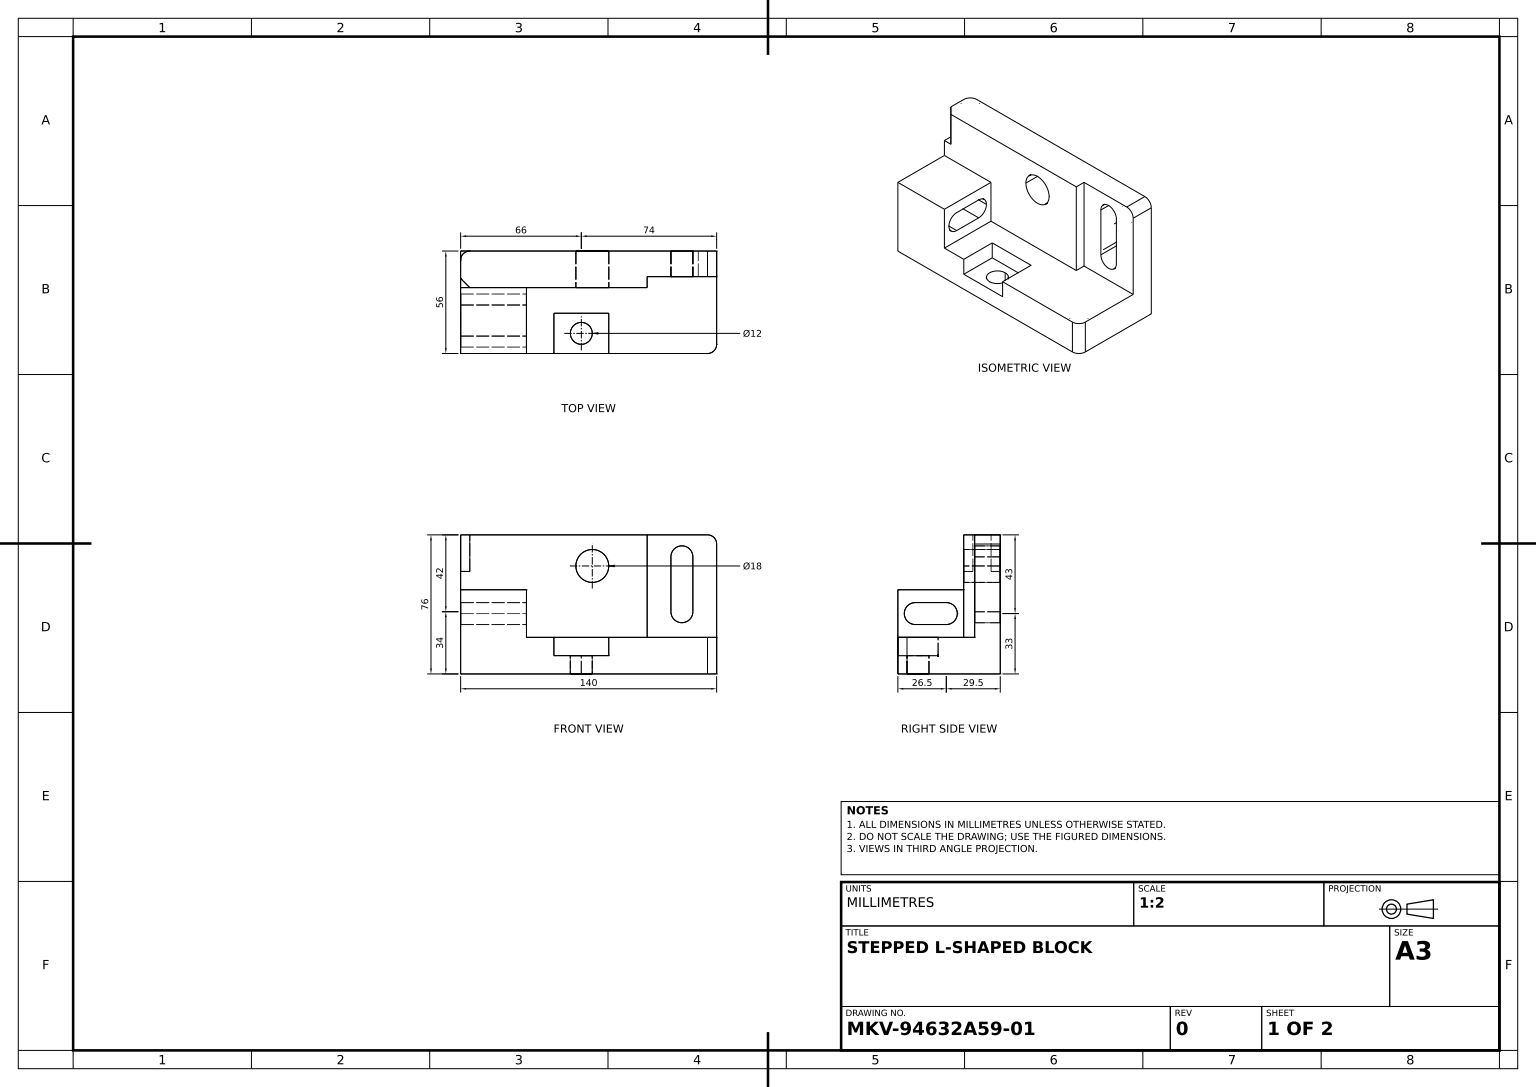
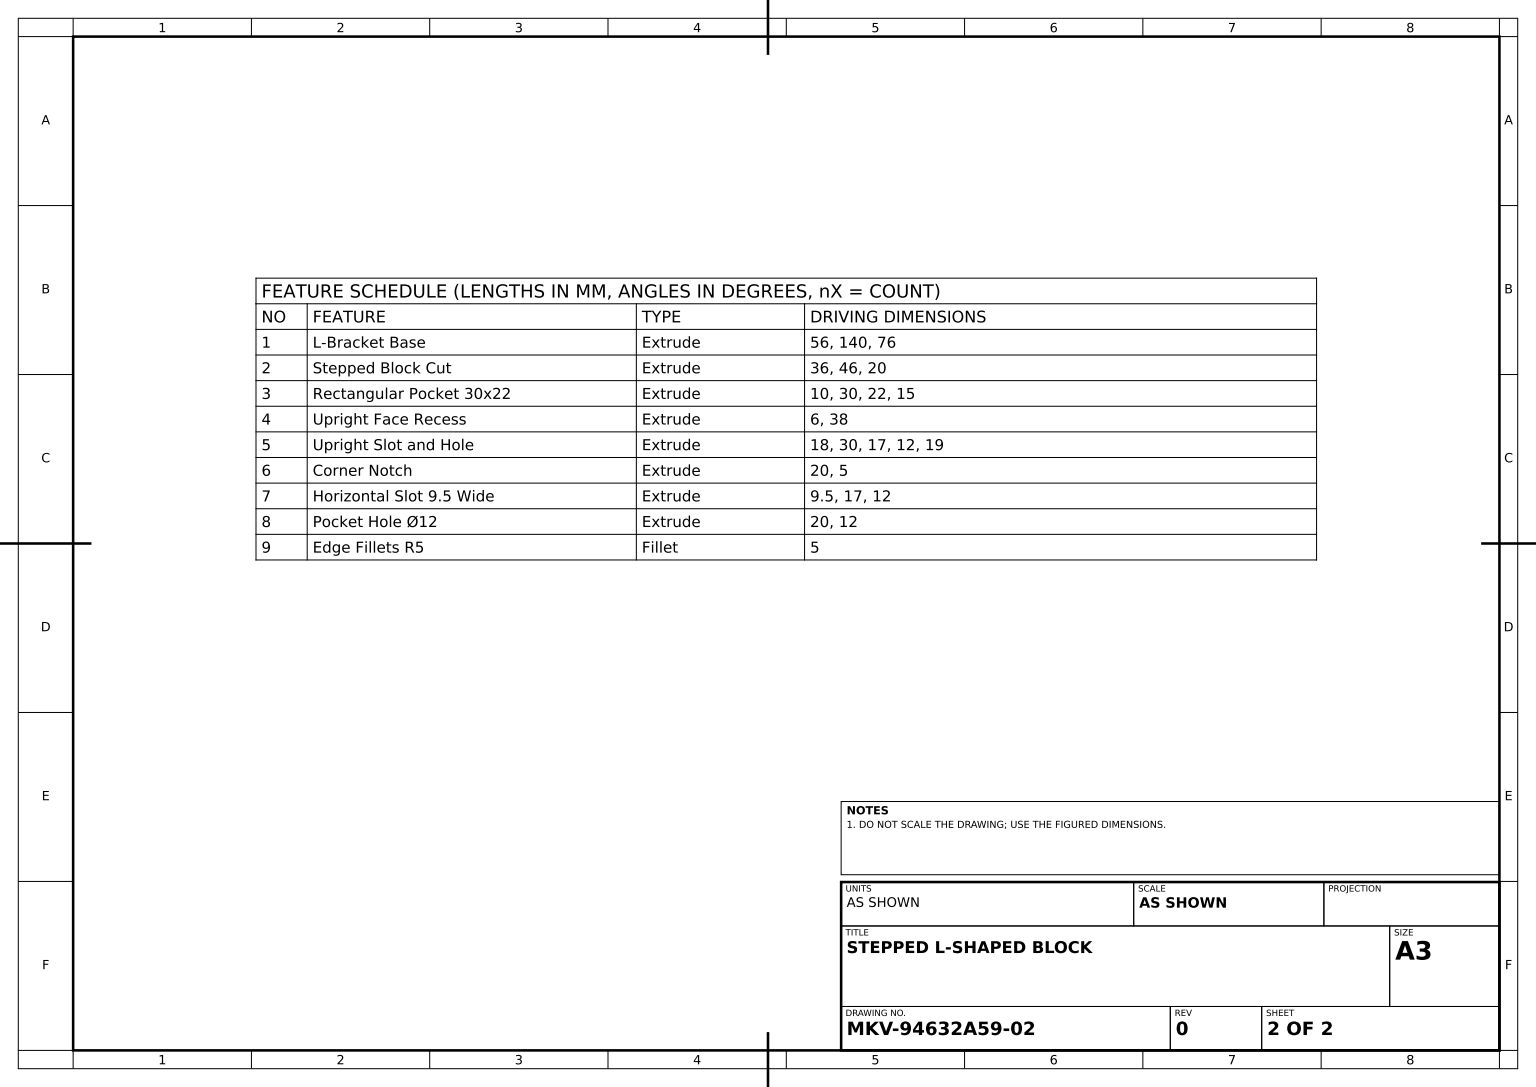
SolidWorks part; units mm, degrees
material "Plain Carbon Steel"
ref_plane "Front Plane" through (0, 0, 0) normal (0, 0, 1) x (1, 0, 0)
ref_plane "Top Plane" through (0, 0, 0) normal (0, 1, 0) x (1, 0, 0)
ref_plane "Right Plane" through (0, 0, 0) normal (1, 0, 0) x (0, 0, -1)
sketch "L-Bracket Profile Sketch" plane through (0, 0, 0) normal (0, 0, 1) x (1, 0, 0)
  line L1 (-70, -38) -> (70, -38)
  line L2 (-70, -38) -> (-70, 38)
  line L3 (-70, 38) -> (70, 38)
  line L4 (70, -38) -> (70, 38)
  line L5 (-70, -38) -> (70, 38) construction
  line L6 (-70, 38) -> (70, -38) construction
  point P0 (0, 0)
  dimension "D1" = 140
  dimension "D2" = 76
extrude "L-Bracket Base" add sketch "L-Bracket Profile Sketch" along normal mid plane 56
sketch "Step Cut Sketch" plane through (0, 0, 28) normal (0, 0, 1) x (1, 0, 0)
  line L0 (-70, 8) -> (-34, 8)
  line L1 (-70, 38) -> (-70, -38) construction
  line L2 (-34, 8) -> (-34, -18)
  line L3 (-34, -18) -> (70, -18)
  line L4 (70, -38) -> (70, 38) construction
  line L5 (70, -18) -> (70, 38)
  line L6 (70, 38) -> (-70, 38)
  line L7 (-70, 38) -> (-70, 8)
  line L8 (-70, -38) -> (70, -38) construction
  dimension "D1" = 46
  dimension "D2" = 36
  dimension "D3" = 20
extrude "Stepped Block Cut" cut sketch "Step Cut Sketch" against normal blind 36
sketch "Rectangular Pocket Sketch" plane through (0, -18, 0) normal (0, 1, 0) x (1, 0, 0)
  line L0 (-34, -28) -> (70, -28) construction
  line L1 (11, -28) -> (-19, -28)
  line L2 (11, -28) -> (11, -6)
  line L3 (11, -6) -> (-19, -6)
  line L4 (-19, -28) -> (-19, -6)
  line L5 (-34, 8) -> (-34, -28) construction
  dimension "D1" = 30
  dimension "D2" = 22
  dimension "D3" = 15
extrude "Rectangular Pocket 30x22" cut sketch "Rectangular Pocket Sketch" against normal blind 10
sketch "Upright Recess Sketch" plane through (0, 0, -8) normal (0, 0, 1) x (1, 0, 0)
  line L0 (11, -18) -> (70, -18) construction
  line L1 (70, 38) -> (32, 38)
  line L2 (70, 38) -> (70, -18)
  line L3 (70, -18) -> (32, -18)
  line L4 (32, 38) -> (32, -18)
  dimension "D1" = 38
extrude "Upright Face Recess" cut sketch "Upright Recess Sketch" against normal blind 6
sketch "Upright Slot and Hole Sketch" plane through (0, 0, -8) normal (0, 0, 1) x (1, 0, 0)
  line L0 (32, 38) -> (32, -18) construction
  line L1 (32, 38) -> (-70, 38) construction
  line L2 (51, -4) -> (51, 26) construction
  line L3 (45, -4) -> (45, 26)
  line L4 (57, -4) -> (57, 26)
  line L5 (70, 38) -> (32, 38) construction
  line L6 (70, -18) -> (70, 38) construction
  circle A0 centre (2, 21) radius 9
  arc A1 (45, -4) -> (57, -4) centre (51, -4) ccw
  arc A2 (57, 26) -> (45, 26) centre (51, 26) ccw
  point P8 (51, 11)
  dimension "D1" = 18
  dimension "D2" = 30
  dimension "D3" = 17
  dimension "D4" = 12
  dimension "D5" = 30
  dimension "D6" = 19
  dimension "D7" = 12
extrude "Upright Slot and Hole" cut sketch "Upright Slot and Hole Sketch" against normal through all
sketch "Corner Notch Sketch" plane through (0, 38, 0) normal (0, 1, 0) x (1, 0, 0)
  line L0 (-70, 13) -> (-65, 8)
  line L1 (-70, 8) -> (-70, 28) construction
  line L2 (-70, 8) -> (-34, 8) construction
  line L4 (70, 28) -> (-70, 28) construction
  line L5 (-70, 13) -> (-70, 8)
  line L6 (-70, 8) -> (-65, 8)
  line L7 (-70, 23) -> (-70, 28)
  line L8 (-70, 28) -> (-65, 28)
  arc A0 (-70, 23) -> (-65, 28) centre (-65, 23) cw
  dimension "D3" = 5
  dimension "D1" = 5
  dimension "D2" = 5
extrude "Corner Notch" cut sketch "Corner Notch Sketch" against normal blind 20
sketch "Horizontal Slot Sketch" plane through (-34, 0, 0) normal (1, 0, 0) x (0, 0, -1)
  line L0 (-18.5, -5) -> (-1.5, -5) construction
  line L1 (-18.5, 1) -> (-1.5, 1)
  line L2 (-18.5, -11) -> (-1.5, -11)
  line L3 (-28, 8) -> (-28, -18) construction
  arc A0 (-18.5, 1) -> (-18.5, -11) centre (-18.5, -5) ccw
  arc A1 (-1.5, -11) -> (-1.5, 1) centre (-1.5, -5) ccw
  point P2 (-10, -5)
  point P9 (-28, -5)
  dimension "D1" = 9.5
  dimension "D2" = 17
  dimension "D3" = 12
extrude "Horizontal Slot 9.5 Wide" cut sketch "Horizontal Slot Sketch" against normal through all
sketch "Pocket Hole Sketch" plane through (0, -28, 0) normal (0, 1, 0) x (1, 0, 0)
  line L0 (11, -6) -> (-19, -6) construction
  line L1 (-19, -6) -> (-19, -28) construction
  circle A0 centre (-4, -17) radius 6
  point P4 (-4, -6)
  point P7 (-19, -17)
  dimension "D1" = 12
extrude "Pocket Hole Ø12" cut sketch "Pocket Hole Sketch" against normal blind 20
fillet "Edge Fillets R5" radius 5 2 edges at (70, 38, -21) (70, -28, 28)
